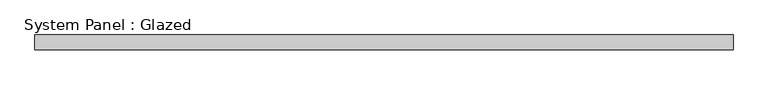
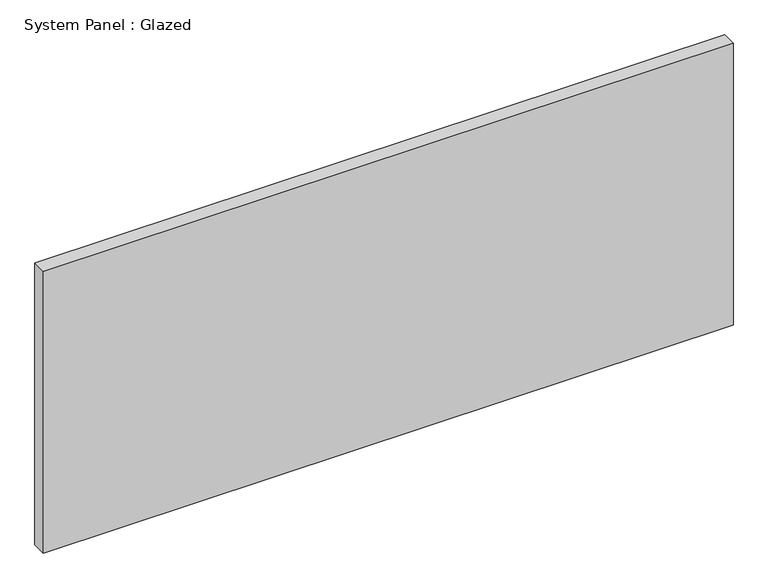
"""IFC4 building model written with IfcOpenShell, lengths in millimetres: plate geometry, System Panel : Glazed."""

from ifc_helpers import new_model, si_unit, origin, origin_with_axes, place, context, project, spatial, polyline, outline, extrude, source, transform, mapped, element, save


def system_panel_glazed_e91e0514(model_context):
    return source(origin(), model_context, "Body", "SweptSolid", [
        extrude(outline(polyline([(595.3125, 19.05), (-595.3125, 19.05), (-595.3125, 44.45), (595.3125, 44.45), (595.3125, 19.05)])), origin_with_axes(), (0.0, 0.0, 1.0), 514.35),
    ])


if __name__ == "__main__":
    model = new_model("IFC4")
    model_context = context("Model", 3, world=origin())
    ifc_project = project(units=[si_unit("LENGTHUNIT", "METRE", prefix="MILLI")], contexts=[model_context])
    site = spatial("IfcSite", under=ifc_project)
    building = spatial("IfcBuilding", under=site)
    placement = place(None, origin())
    system_panel_glazed_shape = system_panel_glazed_e91e0514(model_context)
    element("IfcPlate", 1, ObjectType="System Panel : Glazed", at=placement, inside=building, context=model_context, shape_type="MappedRepresentation", body=[
        mapped(system_panel_glazed_shape, transform((0.0, 0.0, 0.0), x_axis=(1.0, 0.0, 0.0), y_axis=(0.0, 1.0, 0.0), z_axis=(0.0, 0.0, 1.0))),
    ])
    save(model, "model.ifc")

# Revit data of these elements
# Type "System Panel : Glazed"
#   Construction Type Id = "GSP4R"
#   Analytic Construction = "1/8 in Pilkington single glazing"
#   Visual Light Transmittance = 0.9
#   Solar Heat Gain Coefficient = 0.86
#   Heat Transfer Coefficient (U) = 1.18115 BTU/(h·ft²·°F)
# Element 1 (IfcPlate, "System Panel : Glazed")
#   Materials on its faces: "Glass"
# Materials
#   "Glass": class "Glass", colour RGB 0 128 192, transparency 0.75, Description = "Soda Lime Glass", Cost = 0
